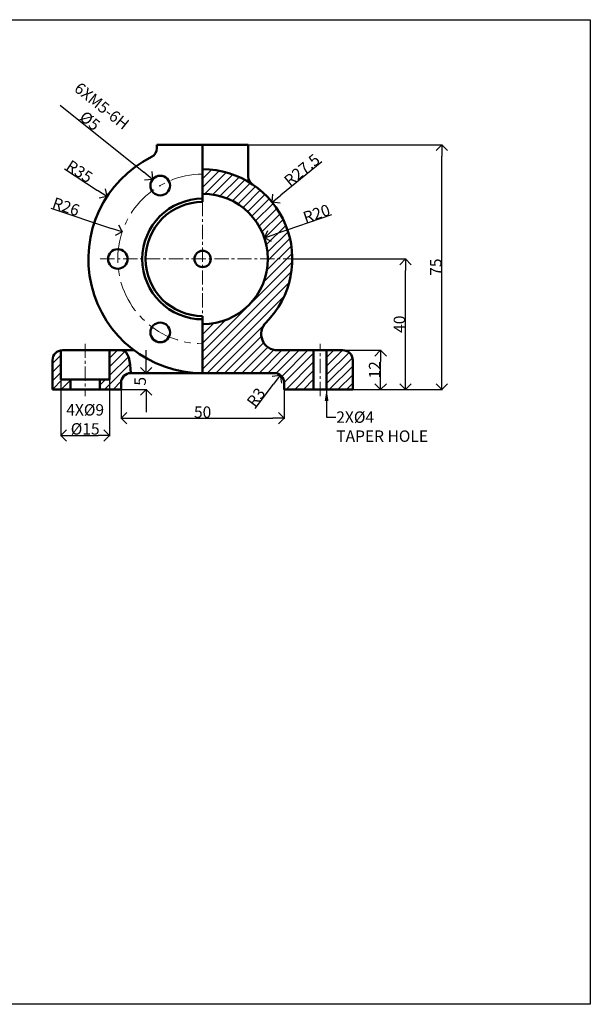
# Model space of a CAD drawing. Units: millimetres. Extents: x 47 to 397, y 26 to 328.
# Tile 2 of 2: x 222 to 397, y 26 to 328. Entities that reach past the tile are written whole.
import ezdxf

# ---------------------------------------------------------------- set-up
doc = ezdxf.new("R2010")
doc.units = ezdxf.units.MM
doc.header["$MEASUREMENT"] = 0
doc.linetypes.add('CENTER', pattern=[2, 1.25, -0.25, 0.25, -0.25])
for name, color, linetype, lineweight in [('M-CNTR', 1, 'CENTER', 18), ('M-DIMS', 2, 'Continuous', 25), ('M-HATC', 8, 'Continuous', 18), ('M-OUTL', 7, 'Continuous', 50), ('M-TEXT', 3, 'Continuous', 25), ('M-TTLB', 7, 'Continuous', 25)]:
    doc.layers.add(name, color=color, linetype=linetype, lineweight=lineweight)
doc.styles.get("Standard").update_dxf_attribs({"font": 'arial.ttf'})
doc.dimstyles.get("Standard").update_dxf_attribs({"dimtxt": 3.5, "dimasz": 3.5, "dimexe": 0.18, "dimexo": 0.0625, "dimgap": 0.09, "dimtad": 1, "dimdec": 0, "dimzin": 0, "dimdsep": 46, "dimtxsty": 'Standard', "dimblk": 'OPEN90', "dimcen": 0.09, "dimclre": 251, "dimadec": 0, "dimazin": 0, "dimtfac": 1, "dimtdec": 0, "dimtofl": 0, "dimtmove": 0, "dimatfit": 3, "dimfxl": 1, "dimtolj": 1, "dimtzin": 0, "dimarcsym": 0})

# ---------------------------------------------------------------- blocks, each defined once
blk = doc.blocks.new('_Open90')
at = {"color": 0, "linetype": 'ByBlock', "lineweight": -2}
for p, q in [((0, 0), (-1, 0)), ((-0.5, 0.5), (0, 0)), ((0, 0), (-0.5, -0.5))]:
    blk.add_line(p, q, dxfattribs=at)
blk = doc.blocks.new('*D22')
at = {"layer": 'Defpoints', "color": 0, "transparency": 16777216}
for p in [(262.79, 279.4), (267.46, 275.64)]:
    blk.add_point(p, dxfattribs=at)
at = {"layer": 'M-DIMS', "color": 0, "lineweight": -2, "transparency": 16777216}
for p, q in [((234.44, 302.19), (260.06, 281.6)), ((265.03, 277.52), (265.21, 277.52)), ((265.12, 277.43), (265.12, 277.61))]:
    blk.add_line(p, q, dxfattribs=at)
at = {"layer": 'M-DIMS', "color": 0, "lineweight": -2, "transparency": 16777216, "xscale": 3.5, "yscale": 3.5, "zscale": 3.5, "rotation": 321.2061599935705}
blk.add_blockref('_Open90', (262.79, 279.4), dxfattribs=at)
at = {"layer": 'M-DIMS', "color": 0, "transparency": 16777216, "insert": (245.4, 299.66), "char_height": 3.5, "attachment_point": 5, "rotation": 321.2062}
blk.add_mtext('\\A1;6XM5-6H\\P%%C5', dxfattribs=at)
blk = doc.blocks.new('*D23')
at = {"layer": 'Defpoints', "color": 0, "transparency": 16777216}
for p in [(248.8, 274.12), (278.12, 255.01)]:
    blk.add_point(p, dxfattribs=at)
at = {"layer": 'M-DIMS', "color": 0, "lineweight": -2, "transparency": 16777216}
for p, q in [((235.76, 282.62), (245.87, 276.03)), ((278.03, 255.01), (278.21, 255.01)), ((278.12, 254.92), (278.12, 255.1))]:
    blk.add_line(p, q, dxfattribs=at)
at = {"layer": 'M-DIMS', "color": 0, "lineweight": -2, "transparency": 16777216, "xscale": 3.5, "yscale": 3.5, "zscale": 3.5, "rotation": 326.9050822797148}
blk.add_blockref('_Open90', (248.8, 274.12), dxfattribs=at)
at = {"layer": 'M-DIMS', "color": 0, "transparency": 16777216, "insert": (240.37, 281.85), "char_height": 3.5, "attachment_point": 5, "rotation": 326.9051}
blk.add_mtext('\\A1;R35', dxfattribs=at)
blk = doc.blocks.new('*D24')
at = {"layer": 'Defpoints', "color": 0, "transparency": 16777216}
for p in [(253.48, 263.29), (278.12, 255.01)]:
    blk.add_point(p, dxfattribs=at)
at = {"layer": 'M-DIMS', "color": 0, "lineweight": -2, "transparency": 16777216}
for p, q in [((231.61, 270.64), (250.16, 264.4)), ((278.03, 255.01), (278.21, 255.01)), ((278.12, 254.92), (278.12, 255.1))]:
    blk.add_line(p, q, dxfattribs=at)
at = {"layer": 'M-DIMS', "color": 0, "lineweight": -2, "transparency": 16777216, "xscale": 3.5, "yscale": 3.5, "zscale": 3.5, "rotation": 341.4250436459752}
blk.add_blockref('_Open90', (253.48, 263.29), dxfattribs=at)
at = {"layer": 'M-DIMS', "color": 0, "transparency": 16777216, "insert": (236.26, 271.06), "char_height": 3.5, "attachment_point": 5, "rotation": 341.425}
blk.add_mtext('\\A1;R26', dxfattribs=at)
blk = doc.blocks.new('*D25')
at = {"layer": 'Defpoints', "color": 0, "transparency": 16777216}
for p in [(299.42, 272.41), (278.12, 255.01)]:
    blk.add_point(p, dxfattribs=at)
at = {"layer": 'M-DIMS', "color": 0, "lineweight": -2, "transparency": 16777216}
for p, q in [((314.63, 284.84), (302.13, 274.62)), ((278.03, 255.01), (278.21, 255.01)), ((278.12, 254.92), (278.12, 255.1))]:
    blk.add_line(p, q, dxfattribs=at)
at = {"layer": 'M-DIMS', "color": 0, "lineweight": -2, "transparency": 16777216, "xscale": 3.5, "yscale": 3.5, "zscale": 3.5, "rotation": 219.2564376675894}
blk.add_blockref('_Open90', (299.42, 272.41), dxfattribs=at)
at = {"layer": 'M-DIMS', "color": 0, "transparency": 16777216, "insert": (308.55, 282.29), "char_height": 3.5, "attachment_point": 5, "rotation": 39.2564}
blk.add_mtext('\\A1;R27.5', dxfattribs=at)
blk = doc.blocks.new('*D26')
at = {"layer": 'Defpoints', "color": 0, "transparency": 16777216}
for p in [(297.05, 261.48), (278.12, 255.01)]:
    blk.add_point(p, dxfattribs=at)
at = {"layer": 'M-DIMS', "color": 0, "lineweight": -2, "transparency": 16777216}
for p, q in [((317.67, 268.53), (300.36, 262.61)), ((278.03, 255.01), (278.21, 255.01)), ((278.12, 254.92), (278.12, 255.1))]:
    blk.add_line(p, q, dxfattribs=at)
at = {"layer": 'M-DIMS', "color": 0, "lineweight": -2, "transparency": 16777216, "xscale": 3.5, "yscale": 3.5, "zscale": 3.5, "rotation": 198.8752853609314}
blk.add_blockref('_Open90', (297.05, 261.48), dxfattribs=at)
at = {"layer": 'M-DIMS', "color": 0, "transparency": 16777216, "insert": (313.03, 268.92), "char_height": 3.5, "attachment_point": 5, "rotation": 18.8753}
blk.add_mtext('\\A1;R20', dxfattribs=at)
blk = doc.blocks.new('*D27')
at = {"layer": 'Defpoints', "color": 0, "transparency": 16777216}
for p in [(234.62, 218.01), (249.62, 218.01), (249.62, 200.88)]:
    blk.add_point(p, dxfattribs=at)
at = {"layer": 'M-DIMS', "color": 0, "lineweight": -2, "transparency": 16777216}
for p, q in [((234.62, 217.95), (234.62, 200.7)), ((249.62, 217.95), (249.62, 200.7)), ((238.12, 200.88), (246.12, 200.88))]:
    blk.add_line(p, q, dxfattribs=at)
at = {"layer": 'M-DIMS', "color": 0, "lineweight": -2, "transparency": 16777216, "xscale": 3.5, "yscale": 3.5, "zscale": 3.5, "rotation": 180}
blk.add_blockref('_Open90', (234.62, 200.88), dxfattribs=at)
at = {"layer": 'M-DIMS', "color": 0, "lineweight": -2, "transparency": 16777216, "xscale": 3.5, "yscale": 3.5, "zscale": 3.5}
blk.add_blockref('_Open90', (249.62, 200.88), dxfattribs=at)
at = {"layer": 'M-DIMS', "color": 0, "transparency": 16777216, "insert": (242.12, 205.83), "char_height": 3.5, "attachment_point": 5}
blk.add_mtext('\\A1;4X%%C9\\P%%C15', dxfattribs=at)
blk = doc.blocks.new('*D28')
at = {"layer": 'Defpoints', "color": 0, "transparency": 16777216}
for p in [(253.12, 215.01), (303.12, 215.01), (303.12, 206.17)]:
    blk.add_point(p, dxfattribs=at)
at = {"layer": 'M-DIMS', "color": 0, "lineweight": -2, "transparency": 16777216}
for p, q in [((253.12, 214.95), (253.12, 205.99)), ((303.12, 214.95), (303.12, 205.99)), ((256.62, 206.17), (299.62, 206.17))]:
    blk.add_line(p, q, dxfattribs=at)
at = {"layer": 'M-DIMS', "color": 0, "lineweight": -2, "transparency": 16777216, "xscale": 3.5, "yscale": 3.5, "zscale": 3.5, "rotation": 180}
blk.add_blockref('_Open90', (253.12, 206.17), dxfattribs=at)
at = {"layer": 'M-DIMS', "color": 0, "lineweight": -2, "transparency": 16777216, "xscale": 3.5, "yscale": 3.5, "zscale": 3.5}
blk.add_blockref('_Open90', (303.12, 206.17), dxfattribs=at)
at = {"layer": 'M-DIMS', "color": 0, "transparency": 16777216, "insert": (278.12, 208.05), "char_height": 3.5, "attachment_point": 5}
blk.add_mtext('\\A1;50', dxfattribs=at)
blk = doc.blocks.new('*D29')
at = {"layer": 'Defpoints', "color": 0, "transparency": 16777216}
for p in [(257.83, 220.01), (260.85, 220.01), (253.12, 215.01)]:
    blk.add_point(p, dxfattribs=at)
at = {"layer": 'M-DIMS', "color": 0, "lineweight": -2, "transparency": 16777216}
for p, q in [((260.85, 223.51), (260.85, 227.01)), ((257.9, 220.01), (261.03, 220.01)), ((253.19, 215.01), (261.03, 215.01)), ((260.85, 211.51), (260.85, 208.01))]:
    blk.add_line(p, q, dxfattribs=at)
at = {"layer": 'M-DIMS', "color": 0, "lineweight": -2, "transparency": 16777216, "xscale": 3.5, "yscale": 3.5, "zscale": 3.5}
for p, rotation in [((260.85, 220.01), 270), ((260.85, 215.01), 90)]:
    blk.add_blockref('_Open90', p, dxfattribs=dict(at, rotation=rotation))
at = {"layer": 'M-DIMS', "color": 0, "transparency": 16777216, "insert": (258.98, 217.51), "char_height": 3.5, "attachment_point": 5, "rotation": 90}
blk.add_mtext('\\A1;5', dxfattribs=at)
blk = doc.blocks.new('*D30')
at = {"layer": 'Defpoints', "color": 0, "transparency": 16777216}
for p in [(301.92, 219.41), (300.12, 217.01)]:
    blk.add_point(p, dxfattribs=at)
at = {"layer": 'M-DIMS', "color": 0, "lineweight": -2, "transparency": 16777216}
blk.add_line((294.24, 209.14), (299.82, 216.61), dxfattribs=at)
at = {"layer": 'M-DIMS', "color": 0, "lineweight": -2, "transparency": 16777216, "xscale": 3.5, "yscale": 3.5, "zscale": 3.5, "rotation": 53.205912704198}
blk.add_blockref('_Open90', (301.92, 219.41), dxfattribs=at)
at = {"layer": 'M-DIMS', "color": 0, "transparency": 16777216, "insert": (294.48, 212.6), "char_height": 3.5, "attachment_point": 5, "rotation": 53.2059}
blk.add_mtext('\\A1;R3', dxfattribs=at)
blk = doc.blocks.new('*D31')
at = {"layer": 'Defpoints', "color": 0, "transparency": 16777216}
for p in [(321.12, 227.01), (332.68, 227.01), (324.12, 215.01)]:
    blk.add_point(p, dxfattribs=at)
at = {"layer": 'M-DIMS', "color": 0, "lineweight": -2, "transparency": 16777216}
for p, q in [((321.19, 227.01), (332.86, 227.01)), ((332.68, 218.51), (332.68, 223.51)), ((324.19, 215.01), (332.86, 215.01))]:
    blk.add_line(p, q, dxfattribs=at)
at = {"layer": 'M-DIMS', "color": 0, "lineweight": -2, "transparency": 16777216, "xscale": 3.5, "yscale": 3.5, "zscale": 3.5}
for p, rotation in [((332.68, 227.01), 90), ((332.68, 215.01), 270)]:
    blk.add_blockref('_Open90', p, dxfattribs=dict(at, rotation=rotation))
at = {"layer": 'M-DIMS', "color": 0, "transparency": 16777216, "insert": (330.84, 221.01), "char_height": 3.5, "attachment_point": 5, "rotation": 90}
blk.add_mtext('\\A1;12', dxfattribs=at)
blk = doc.blocks.new('*D32')
at = {"layer": 'Defpoints', "color": 0, "transparency": 16777216}
for p in [(305.62, 255.01), (340.32, 255.01), (324.12, 215.01)]:
    blk.add_point(p, dxfattribs=at)
at = {"layer": 'M-DIMS', "color": 0, "lineweight": -2, "transparency": 16777216}
for p, q in [((305.69, 255.01), (340.5, 255.01)), ((340.32, 218.51), (340.32, 251.51)), ((324.19, 215.01), (340.5, 215.01))]:
    blk.add_line(p, q, dxfattribs=at)
at = {"layer": 'M-DIMS', "color": 0, "lineweight": -2, "transparency": 16777216, "xscale": 3.5, "yscale": 3.5, "zscale": 3.5}
for p, rotation in [((340.32, 255.01), 90), ((340.32, 215.01), 270)]:
    blk.add_blockref('_Open90', p, dxfattribs=dict(at, rotation=rotation))
at = {"layer": 'M-DIMS', "color": 0, "transparency": 16777216, "insert": (338.44, 235.01), "char_height": 3.5, "attachment_point": 5, "rotation": 90}
blk.add_mtext('\\A1;40', dxfattribs=at)
blk = doc.blocks.new('*D33')
at = {"layer": 'Defpoints', "color": 0, "transparency": 16777216}
for p in [(292.12, 290.01), (351.44, 290.01), (324.12, 215.01)]:
    blk.add_point(p, dxfattribs=at)
at = {"layer": 'M-DIMS', "color": 0, "lineweight": -2, "transparency": 16777216}
for p, q in [((292.19, 290.01), (351.62, 290.01)), ((351.44, 218.51), (351.44, 286.51)), ((324.19, 215.01), (351.62, 215.01))]:
    blk.add_line(p, q, dxfattribs=at)
at = {"layer": 'M-DIMS', "color": 0, "lineweight": -2, "transparency": 16777216, "xscale": 3.5, "yscale": 3.5, "zscale": 3.5}
for p, rotation in [((351.44, 290.01), 90), ((351.44, 215.01), 270)]:
    blk.add_blockref('_Open90', p, dxfattribs=dict(at, rotation=rotation))
at = {"layer": 'M-DIMS', "color": 0, "transparency": 16777216, "insert": (349.57, 252.51), "char_height": 3.5, "attachment_point": 5, "rotation": 90}
blk.add_mtext('\\A1;75', dxfattribs=at)

msp = doc.modelspace()

# ---------------------------------------------------------------- hatches: boundary and pattern name
at = {"layer": 'M-HATC'}
h = msp.add_hatch(dxfattribs=at)
h.set_pattern_fill('ANSI31', color=256, scale=15)
h.set_pattern_definition([(45, (9.835, -468.6345), (-1.325825, 1.325825), [])])
edge = h.paths.add_edge_path()
edge.add_spline(control_points=[(256.12, 220.01), (255.88, 223.45), (255.65, 226.88), (253.2, 227.01)], knot_values=[0, 0, 0, 0, 7.586741, 7.586741, 7.586741, 7.586741], degree=3, periodic=0)
edge.add_line((253.2, 227.01), (249.62, 227.01))
edge.add_line((249.62, 227.01), (249.62, 218.01))
edge.add_line((249.62, 218.01), (246.62, 218.01))
edge.add_line((246.62, 218.01), (246.62, 215.01))
edge.add_line((246.62, 215.01), (253.12, 215.01))
edge.add_line((253.12, 215.01), (253.12, 217.01))
edge.add_arc((256.12, 217.01), 3, 90, 180, ccw=False)
h.paths.add_polyline_path([(237.62, 218.01), (234.62, 218.01), (234.62, 226.97, 0.365977), (232.12, 224.01), (232.12, 215.01), (237.62, 215.01)])
h.paths.add_polyline_path([(312.12, 227.01), (301.09, 227.01, -0.668478), (297.55, 235.55, 0.199128), (305.62, 255.01), (298.12, 255.01, -0.414214), (278.12, 235.01), (278.12, 220.01), (300.12, 220.01, -0.414214), (303.12, 217.01), (303.12, 215.01), (312.12, 215.01)])
h.paths.add_polyline_path([(324.12, 224.01, 0.414214), (321.12, 227.01), (316.12, 227.01), (316.12, 215.01), (324.12, 215.01)])
h.paths.add_polyline_path([(278.12, 282.51), (278.12, 275.01, -0.414214), (298.12, 255.01), (305.62, 255.01, 0.414214)])

# ---------------------------------------------------------------- linework, layer by layer
at = {"layer": 'M-CNTR', "ltscale": 3.5}
for p, q in [((278.12, 272.51), (278.12, 237.51)), ((246.76, 255.01), (306.68, 255.01)), ((242.12, 229.03), (242.12, 212.99)), ((314.12, 212.99), (314.12, 229.03))]:
    msp.add_line(p, q, dxfattribs=at)
at = {"layer": 'M-CNTR', "ltscale": 8}
msp.add_arc((278.12, 255.01), 26, 90, 270, dxfattribs=at)
at = {"layer": 'M-OUTL'}
for p, q in [((264.12, 290.01), (292.12, 290.01)), ((264.12, 290.01), (264.12, 288.99)), ((278.12, 290.01), (278.12, 272.51)), ((292.12, 290.01), (292.12, 280.33)), ((278.12, 237.51), (278.12, 220.01)), ((234.62, 227.01), (234.62, 218.01)), ((235.12, 227.01), (257.12, 227.01)), ((249.62, 227.01), (249.62, 218.01)), ((301.09, 227.01), (321.12, 227.01)), ((312.12, 227.01), (312.12, 215.01)), ((316.12, 227.01), (316.12, 215.01)), ((232.12, 224.01), (232.12, 215.01)), ((324.12, 224.01), (324.12, 215.01)), ((234.62, 218.01), (249.62, 218.01)), ((237.62, 215.01), (237.62, 218.01)), ((237.62, 218.01), (237.62, 215.01)), ((246.62, 215.01), (246.62, 218.01)), ((256.12, 220.01), (300.12, 220.01)), ((232.12, 215.01), (253.12, 215.01)), ((253.12, 217.01), (253.12, 215.01)), ((303.12, 217.01), (303.12, 215.01)), ((303.12, 215.01), (324.12, 215.01))]:
    msp.add_line(p, q, dxfattribs=at)
for centre, radius in [((265.12, 277.52), 3), ((252.12, 255.01), 3), ((278.12, 255.01), 2.5), ((265.12, 232.49), 3)]:
    msp.add_circle(centre, radius, dxfattribs=at)
for centre, radius, start, end in [((261.12, 288.99), 3, 296.575, 0), ((278.12, 255.01), 35, 116.575, 270), ((278.12, 255.01), 27.5, 314.9525, 90), ((295.12, 280.33), 3, 180, 236.1254), ((278.12, 255.01), 20, 270, 90), ((278.12, 255.01), 18.5, 90, 270), ((278.12, 255.01), 17.5, 90, 270), ((301.09, 232.01), 5, 134.9525, 270), ((235.12, 224.01), 3, 90, 180), ((321.12, 224.01), 3, 0, 90), ((256.12, 217.01), 3, 90, 180), ((300.12, 217.01), 3, 0, 90)]:
    msp.add_arc(centre, radius, start, end, dxfattribs=at)
msp.add_open_spline([(256.12, 220.01), (255.88, 223.45), (255.63, 227.08), (252.92, 227.01), (252.78, 227.01)], degree=3, knots=[0, 0, 0, 0, 7.586741, 8.010074, 8.010074, 8.010074, 8.010074], dxfattribs=at)
at = {"layer": 'M-TTLB'}
msp.add_lwpolyline([(47.15, 328.38), (396.95, 328.38), (396.95, 26.47), (47.15, 26.47)], close=True, dxfattribs=at)

# ---------------------------------------------------------------- texts
at = {"layer": 'M-TEXT', "insert": (319.09, 208.27), "char_height": 3.5, "attachment_point": 1}
msp.add_mtext('2X%%C4\\PTAPER HOLE', dxfattribs=at)

# ---------------------------------------------------------------- dimensions: what is measured, and where the dimension line sits
at = {"layer": 'M-DIMS'}
dim = msp.add_diameter_dim_2p(p1=(267.46, 275.64), p2=(262.79, 279.4), text='6XM5-6H\\P%%C5', dimstyle='Standard', override={"dimclrd": 0, "dimclre": 0, "dimclrt": 0}, dxfattribs=at)
dim.commit()
dim.dimension.update_dxf_attribs({"geometry": '*D22', "text_midpoint": (242.33, 295.85), "dimtype": 163})
for base, p1, p2, picture, middle in [((351.44, 290.01), (324.12, 215.01), (292.12, 290.01), '*D33', (349.57, 252.51)), ((340.32, 255.01), (324.12, 215.01), (305.62, 255.01), '*D32', (338.44, 235.01)), ((260.85, 220.01), (253.12, 215.01), (257.83, 220.01), '*D29', (258.98, 217.51)), ((332.68, 227.01), (324.12, 215.01), (321.12, 227.01), '*D31', (330.84, 221.01))]:
    dim = msp.add_linear_dim(base=base, p1=p1, p2=p2, angle=90, dimstyle='Standard', override={"dimclrd": 0, "dimclre": 0, "dimclrt": 0}, dxfattribs=at)
    dim.commit()
    dim.dimension.update_dxf_attribs({"geometry": picture, "text_midpoint": middle})
for mpoint, override, picture, middle in [((299.42, 272.41), {"dimdec": 1, "dimclrd": 0, "dimclre": 0, "dimclrt": 0}, '*D25', (308.55, 282.29)), ((248.8, 274.12), {"dimclrd": 0, "dimclre": 0, "dimclrt": 0}, '*D23', (240.37, 281.85))]:
    dim = msp.add_radius_dim(center=(278.12, 255.01), mpoint=mpoint, dimstyle='Standard', override=override, dxfattribs=at)
    dim.commit()
    dim.dimension.update_dxf_attribs({"geometry": picture, "text_midpoint": middle})
for center, mpoint, picture, middle in [((278.12, 255.01), (253.48, 263.29), '*D24', (235.66, 269.28)), ((278.12, 255.01), (297.05, 261.48), '*D26', (313.63, 267.15)), ((300.12, 217.01), (301.92, 219.41), '*D30', (295.98, 211.47))]:
    dim = msp.add_radius_dim(center=center, mpoint=mpoint, dimstyle='Standard', override={"dimclrd": 0, "dimclre": 0, "dimclrt": 0}, dxfattribs=at)
    dim.commit()
    dim.dimension.update_dxf_attribs({"geometry": picture, "text_midpoint": middle, "dimtype": 164})
dim = msp.add_linear_dim(base=(249.62, 200.88), p1=(234.62, 218.01), p2=(249.62, 218.01), text='4X%%C9\\P%%C<>', dimstyle='Standard', override={"dimclrd": 0, "dimclre": 0, "dimclrt": 0}, dxfattribs=at)
dim.commit()
dim.dimension.update_dxf_attribs({"geometry": '*D27', "text_midpoint": (242.12, 205.83)})
dim = msp.add_linear_dim(base=(303.12, 206.17), p1=(253.12, 215.01), p2=(303.12, 215.01), dimstyle='Standard', override={"dimclrd": 0, "dimclre": 0, "dimclrt": 0}, dxfattribs=at)
dim.commit()
dim.dimension.update_dxf_attribs({"geometry": '*D28', "text_midpoint": (278.12, 208.05)})

# ---------------------------------------------------------------- leaders
at = {"layer": 'M-DIMS', "annotation_type": 0, "has_hookline": 1, "hookline_direction": 1, "text_width": 30.6}
msp.add_leader([(316.12, 215.01), (316.12, 206.52), (319, 206.52)], dimstyle='Standard', override={"dimgap": 0.09, "dimtad": 0}, dxfattribs=at)

doc.saveas('drawing.dxf')
